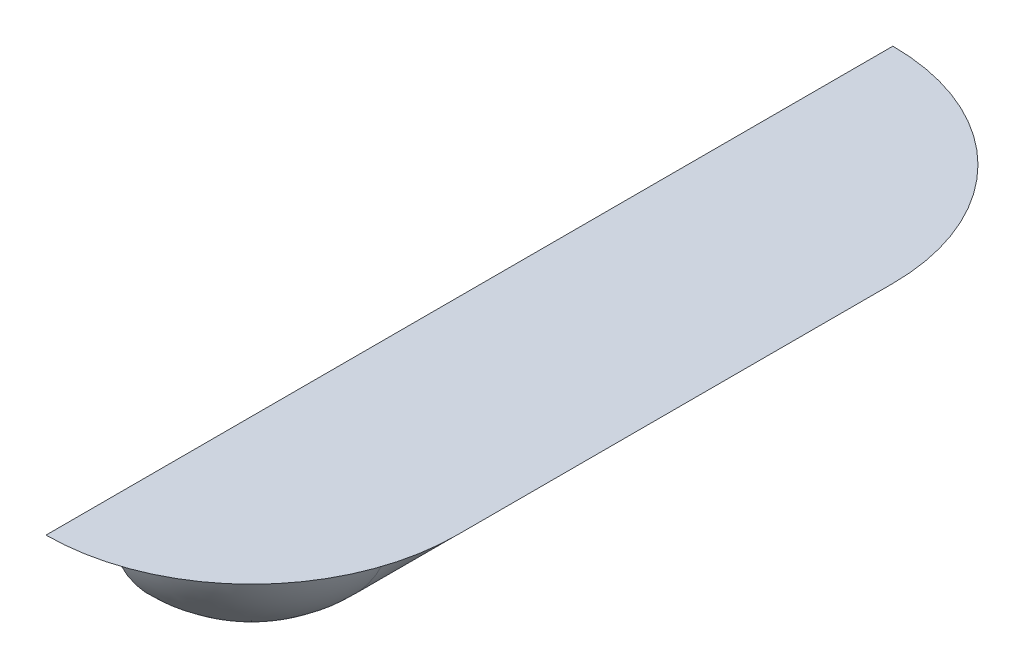
from build123d import *

# Parameters (mm, degrees)
BASE_PROFILE_SKETCH_W          = 50
BASE_PROFILE_SKETCH_H          = 3.464243611
BASE_EXTRUSION_150_DEPTH       = 75
LOUVER_BOSS_DEPTH              = 30
UPPER_CURL_REVOLVE_90DEG_ANGLE = 90
LOWER_CURL_REVOLVE_90DEG_ANGLE = 90
BOTTOM_FILLET_R10_R            = 10
TRIM_CUT_PROFILE_W             = 150
TRIM_CUT_PROFILE_H             = 3.464243611
LOUVER_TRIM_CUT_DEPTH          = 93.33092672


with BuildPart() as part:
    # Base Profile Sketch → Base Extrusion 150 (new, symmetric)
    with BuildSketch(Plane.XY):
        with Locations((0, 1.732121806)):
            Rectangle(BASE_PROFILE_SKETCH_W, BASE_PROFILE_SKETCH_H)
    extrude(amount=BASE_EXTRUSION_150_DEPTH, both=True)

    # Louver Body → Louver Boss (add, symmetric)
    with BuildSketch(Plane.XY):
        with BuildLine():
            Line((-10, 0), (-10, -20))
            ThreePointArc((-10, -20), (4.142135624, -14.142135624), (10, 0))
            Line((10, 0), (-10, 0))
        make_face()
    extrude(amount=LOUVER_BOSS_DEPTH, both=True)

    # Upper Curl Profile → Upper Curl Revolve 90deg (revolve)
    with BuildSketch(Plane.XY.offset(30)):
        with BuildLine():
            Line((10, 0), (-10, 0))
            Line((-10, 0), (-10, -20))
            ThreePointArc((-10, -20), (4.142135624, -14.142135624), (10, 0))
        make_face()
    revolve(axis=Axis((-10, 0, 30), (0, -1, 0)), revolution_arc=UPPER_CURL_REVOLVE_90DEG_ANGLE)

    # Lower Curl Profile → Lower Curl Revolve 90deg (revolve)
    with BuildSketch(Plane(origin=(0, 0, -30), x_dir=(-1, 0, 0), z_dir=(0, 0, -1))):
        with BuildLine():
            Line((10, 0), (-10, 0))
            ThreePointArc((-10, 0), (-4.142135624, -14.142135624), (10, -20))
            Line((10, -20), (10, 0))
        make_face()
    revolve(axis=Axis((-10, -20, -30), (0, 1, 0)), revolution_arc=LOWER_CURL_REVOLVE_90DEG_ANGLE)

    # Bottom Fillet R10
    bottom_fillet_r10_edges = [part.edges().sort_by_distance(p)[0] for p in [
        (10, 0, 0),
        (4.142135624, 0, 44.142135624),
        (4.142135624, 0, -44.142135624),
    ]]
    fillet(bottom_fillet_r10_edges, radius=BOTTOM_FILLET_R10_R)

    # Trim Cut Profile → Louver Trim Cut (cut, through all)
    with BuildSketch(Plane.ZY.offset(25)):
        with Locations((0, 1.732121806)):
            Rectangle(TRIM_CUT_PROFILE_W, TRIM_CUT_PROFILE_H)
    extrude(amount=-LOUVER_TRIM_CUT_DEPTH, mode=Mode.SUBTRACT)


solid = part.part
